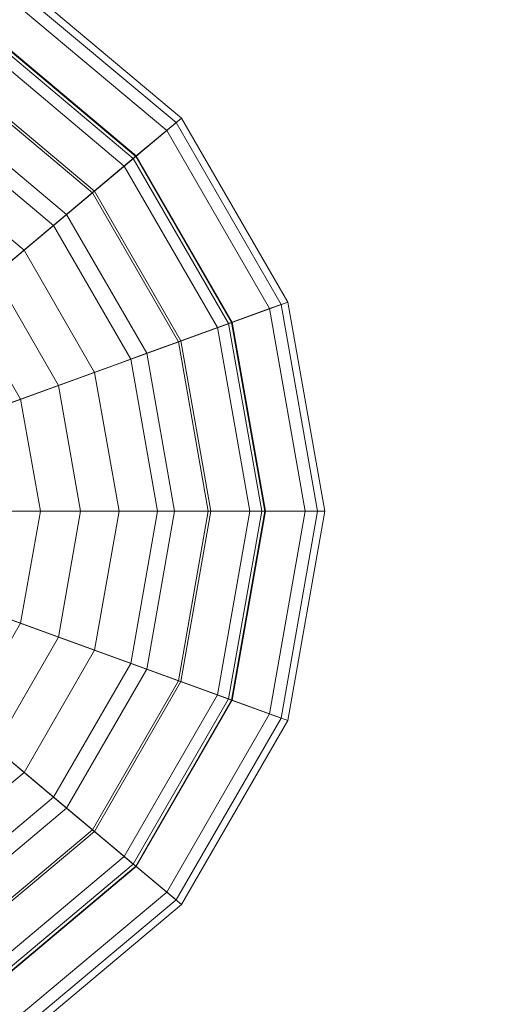
# Model space of a CAD drawing. Units: inches. Extents: x 375 to 1122, y 27 to 1069.
# Tile 142 of 155: x 733.741 to 734.829, y 898.026 to 900.205. Entities that reach past the tile are written whole.
import ezdxf

# ---------------------------------------------------------------- set-up
doc = ezdxf.new("R2010")
doc.units = ezdxf.units.IN
doc.layers.add('A-ANNO-DIMS', color=2, linetype='Continuous', lineweight=18)
doc.layers.add('Furniture', color=30, linetype='Continuous', lineweight=18)
doc.styles.get("Standard").update_dxf_attribs({"font": 'arial.ttf'})
doc.dimstyles.new('ISO-25', dxfattribs={"dimtxt": 12, "dimasz": 2.5, "dimexe": 1.5, "dimexo": 1.5, "dimtad": 1, "dimdec": 1, "dimlunit": 3, "dimtxsty": 'Standard', "dimblk": 'ARCHTICK', "dimcen": 2.5, "dimadec": 0, "dimazin": 0, "dimtfac": 1, "dimtdec": 1, "dimtmove": 0, "dimatfit": 3, "dimfxl": 1.5, "dimfxlon": 1, "dimarcsym": 0})

# ---------------------------------------------------------------- blocks, each defined once
blk = doc.blocks.new('A$C403C54AD')
for points in [[(0.980157, 1.23678, -0.04658), (0.980157, 1.202917, -0.043501), (0.980157, 1.202917, -0.043501), (0.968576, 1.234737, -0.04658)], [(0.980157, 1.233514, -0.043349), (0.980157, 1.23678, -0.04658), (0.968576, 1.234737, -0.04658), (0.969693, 1.231669, -0.043349)], [(0.991739, 1.234737, -0.04658), (0.980157, 1.202917, -0.043501), (0.980157, 1.202917, -0.043501), (0.980157, 1.23678, -0.04658)], [(0.990622, 1.231669, -0.043349), (0.991739, 1.234737, -0.04658), (0.980157, 1.23678, -0.04658), (0.980157, 1.233514, -0.043349)], [(0.980157, 1.233473, 0.116404), (0.980157, 1.236381, 0.10318), (0.968712, 1.234363, 0.10318), (0.969706, 1.231631, 0.116404)], [(0.980157, 1.236381, 0.10318), (0.980157, 1.235706, 0.074938), (0.968943, 1.233728, 0.074938), (0.968712, 1.234363, 0.10318)], [(0.990608, 1.231631, 0.116404), (0.991602, 1.234363, 0.10318), (0.980157, 1.236381, 0.10318), (0.980157, 1.233473, 0.116404)], [(0.991602, 1.234363, 0.10318), (0.991372, 1.233728, 0.074938), (0.980157, 1.235706, 0.074938), (0.980157, 1.236381, 0.10318)], [(0.980157, 1.235706, 0.074938), (0.980157, 1.230341, 0.056929), (0.970778, 1.228687, 0.056929), (0.968943, 1.233728, 0.074938)], [(0.991372, 1.233728, 0.074938), (0.989537, 1.228687, 0.056929), (0.980157, 1.230341, 0.056929), (0.980157, 1.235706, 0.074938)], [(0.968576, 1.234737, -0.04658), (0.980157, 1.202917, -0.043501), (0.980157, 1.202917, -0.043501), (0.958391, 1.228857, -0.04658)], [(0.969693, 1.231669, -0.043349), (0.968576, 1.234737, -0.04658), (0.958391, 1.228857, -0.04658), (0.96049, 1.226356, -0.043349)], [(1.001923, 1.228857, -0.04658), (0.980157, 1.202917, -0.043501), (0.980157, 1.202917, -0.043501), (0.991739, 1.234737, -0.04658)], [(0.999824, 1.226356, -0.043349), (1.001923, 1.228857, -0.04658), (0.991739, 1.234737, -0.04658), (0.990622, 1.231669, -0.043349)], [(0.969706, 1.231631, 0.116404), (0.968712, 1.234363, 0.10318), (0.958647, 1.228552, 0.10318), (0.960516, 1.226325, 0.116404)], [(0.968712, 1.234363, 0.10318), (0.968943, 1.233728, 0.074938), (0.959081, 1.228035, 0.074938), (0.958647, 1.228552, 0.10318)], [(0.999798, 1.226325, 0.116404), (1.001667, 1.228552, 0.10318), (0.991602, 1.234363, 0.10318), (0.990608, 1.231631, 0.116404)], [(1.001667, 1.228552, 0.10318), (1.001233, 1.228035, 0.074938), (0.991372, 1.233728, 0.074938), (0.991602, 1.234363, 0.10318)], [(0.968943, 1.233728, 0.074938), (0.970778, 1.228687, 0.056929), (0.96253, 1.223925, 0.056929), (0.959081, 1.228035, 0.074938)], [(0.980157, 1.217132, -0.040074), (0.980157, 1.233514, -0.043349), (0.969693, 1.231669, -0.043349), (0.975296, 1.216274, -0.040074)], [(0.980157, 1.228477, 0.12581), (0.980157, 1.233473, 0.116404), (0.969706, 1.231631, 0.116404), (0.971415, 1.226936, 0.12581)], [(0.980157, 1.233296, 0.102963), (0.980157, 1.230487, 0.115599), (0.970728, 1.228824, 0.115599), (0.969767, 1.231464, 0.102963)], [(0.980157, 1.232638, 0.075423), (0.980157, 1.233296, 0.102963), (0.969767, 1.231464, 0.102963), (0.969992, 1.230846, 0.075423)], [(0.985019, 1.216274, -0.040074), (0.990622, 1.231669, -0.043349), (0.980157, 1.233514, -0.043349), (0.980157, 1.217132, -0.040074)], [(0.988899, 1.226936, 0.12581), (0.990608, 1.231631, 0.116404), (0.980157, 1.233473, 0.116404), (0.980157, 1.228477, 0.12581)], [(0.990547, 1.231464, 0.102963), (0.989586, 1.228824, 0.115599), (0.980157, 1.230487, 0.115599), (0.980157, 1.233296, 0.102963)], [(0.990322, 1.230846, 0.075423), (0.990547, 1.231464, 0.102963), (0.980157, 1.233296, 0.102963), (0.980157, 1.232638, 0.075423)], [(1.001233, 1.228035, 0.074938), (0.997785, 1.223925, 0.056929), (0.989537, 1.228687, 0.056929), (0.991372, 1.233728, 0.074938)], [(0.980157, 1.227531, 0.058276), (0.980157, 1.232638, 0.075423), (0.969992, 1.230846, 0.075423), (0.971739, 1.226046, 0.058276)], [(0.988575, 1.226046, 0.058276), (0.990322, 1.230846, 0.075423), (0.980157, 1.232638, 0.075423), (0.980157, 1.227531, 0.058276)], [(0.975296, 1.216274, -0.040074), (0.969693, 1.231669, -0.043349), (0.96049, 1.226356, -0.043349), (0.971021, 1.213806, -0.040074)], [(0.989294, 1.213806, -0.040074), (0.999824, 1.226356, -0.043349), (0.990622, 1.231669, -0.043349), (0.985019, 1.216274, -0.040074)], [(0.971415, 1.226936, 0.12581), (0.969706, 1.231631, 0.116404), (0.960516, 1.226325, 0.116404), (0.963728, 1.222497, 0.12581)], [(0.969767, 1.231464, 0.102963), (0.970728, 1.228824, 0.115599), (0.962436, 1.224037, 0.115599), (0.96063, 1.226189, 0.102963)], [(0.969992, 1.230846, 0.075423), (0.969767, 1.231464, 0.102963), (0.96063, 1.226189, 0.102963), (0.961053, 1.225685, 0.075423)], [(0.996587, 1.222497, 0.12581), (0.999798, 1.226325, 0.116404), (0.990608, 1.231631, 0.116404), (0.988899, 1.226936, 0.12581)], [(0.999684, 1.226189, 0.102963), (0.997878, 1.224037, 0.115599), (0.989586, 1.228824, 0.115599), (0.990547, 1.231464, 0.102963)], [(0.999261, 1.225685, 0.075423), (0.999684, 1.226189, 0.102963), (0.990547, 1.231464, 0.102963), (0.990322, 1.230846, 0.075423)], [(0.971739, 1.226046, 0.058276), (0.969992, 1.230846, 0.075423), (0.961053, 1.225685, 0.075423), (0.964336, 1.221772, 0.058276)], [(0.995978, 1.221772, 0.058276), (0.999261, 1.225685, 0.075423), (0.990322, 1.230846, 0.075423), (0.988575, 1.226046, 0.058276)], [(0.980157, 1.230487, 0.115599), (0.980157, 1.225399, 0.12581), (0.972468, 1.224043, 0.12581), (0.970728, 1.228824, 0.115599)], [(0.980157, 1.230341, 0.056929), (0.980157, 1.223275, 0.046697), (0.973195, 1.222047, 0.046697), (0.970778, 1.228687, 0.056929)], [(0.989586, 1.228824, 0.115599), (0.987846, 1.224043, 0.12581), (0.980157, 1.225399, 0.12581), (0.980157, 1.230487, 0.115599)], [(0.989537, 1.228687, 0.056929), (0.98712, 1.222047, 0.046697), (0.980157, 1.223275, 0.046697), (0.980157, 1.230341, 0.056929)], [(0.958391, 1.228857, -0.04658), (0.980157, 1.202917, -0.043501), (0.980157, 1.202917, -0.043501), (0.950832, 1.219849, -0.04658)], [(0.96049, 1.226356, -0.043349), (0.958391, 1.228857, -0.04658), (0.950832, 1.219849, -0.04658), (0.95366, 1.218216, -0.043349)], [(0.960516, 1.226325, 0.116404), (0.958647, 1.228552, 0.10318), (0.951177, 1.219649, 0.10318), (0.953695, 1.218195, 0.116404)], [(0.958647, 1.228552, 0.10318), (0.959081, 1.228035, 0.074938), (0.951762, 1.219312, 0.074938), (0.951177, 1.219649, 0.10318)], [(0.970728, 1.228824, 0.115599), (0.972468, 1.224043, 0.12581), (0.965707, 1.220139, 0.12581), (0.962436, 1.224037, 0.115599)], [(0.970778, 1.228687, 0.056929), (0.973195, 1.222047, 0.046697), (0.967072, 1.218512, 0.046697), (0.96253, 1.223925, 0.056929)], [(0.980157, 1.225399, 0.12581), (0.980157, 1.228477, 0.12581), (0.971415, 1.226936, 0.12581), (0.972468, 1.224043, 0.12581)], [(1.009483, 1.219849, -0.04658), (0.980157, 1.202917, -0.043501), (0.980157, 1.202917, -0.043501), (1.001923, 1.228857, -0.04658)], [(0.987846, 1.224043, 0.12581), (0.988899, 1.226936, 0.12581), (0.980157, 1.228477, 0.12581), (0.980157, 1.225399, 0.12581)], [(0.997785, 1.223925, 0.056929), (0.993243, 1.218512, 0.046697), (0.98712, 1.222047, 0.046697), (0.989537, 1.228687, 0.056929)], [(0.997878, 1.224037, 0.115599), (0.994608, 1.220139, 0.12581), (0.987846, 1.224043, 0.12581), (0.989586, 1.228824, 0.115599)], [(1.00662, 1.218195, 0.116404), (1.009137, 1.219649, 0.10318), (1.001667, 1.228552, 0.10318), (0.999798, 1.226325, 0.116404)], [(1.006655, 1.218216, -0.043349), (1.009483, 1.219849, -0.04658), (1.001923, 1.228857, -0.04658), (0.999824, 1.226356, -0.043349)], [(1.009137, 1.219649, 0.10318), (1.008553, 1.219312, 0.074938), (1.001233, 1.228035, 0.074938), (1.001667, 1.228552, 0.10318)], [(0.959081, 1.228035, 0.074938), (0.96253, 1.223925, 0.056929), (0.956408, 1.216629, 0.056929), (0.951762, 1.219312, 0.074938)], [(1.008553, 1.219312, 0.074938), (1.003907, 1.216629, 0.056929), (0.997785, 1.223925, 0.056929), (1.001233, 1.228035, 0.074938)], [(0.980157, 1.221045, 0.048884), (0.980157, 1.227531, 0.058276), (0.971739, 1.226046, 0.058276), (0.973957, 1.219951, 0.048884)], [(0.986357, 1.219951, 0.048884), (0.988575, 1.226046, 0.058276), (0.980157, 1.227531, 0.058276), (0.980157, 1.221045, 0.048884)], [(0.972468, 1.224043, 0.12581), (0.971415, 1.226936, 0.12581), (0.963728, 1.222497, 0.12581), (0.965707, 1.220139, 0.12581)], [(0.994608, 1.220139, 0.12581), (0.996587, 1.222497, 0.12581), (0.988899, 1.226936, 0.12581), (0.987846, 1.224043, 0.12581)], [(0.971021, 1.213806, -0.040074), (0.96049, 1.226356, -0.043349), (0.95366, 1.218216, -0.043349), (0.967847, 1.210025, -0.040074)], [(0.963728, 1.222497, 0.12581), (0.960516, 1.226325, 0.116404), (0.953695, 1.218195, 0.116404), (0.958022, 1.215697, 0.12581)], [(0.992467, 1.210025, -0.040074), (1.006655, 1.218216, -0.043349), (0.999824, 1.226356, -0.043349), (0.989294, 1.213806, -0.040074)], [(1.002293, 1.215697, 0.12581), (1.00662, 1.218195, 0.116404), (0.999798, 1.226325, 0.116404), (0.996587, 1.222497, 0.12581)], [(0.96063, 1.226189, 0.102963), (0.962436, 1.224037, 0.115599), (0.956282, 1.216702, 0.115599), (0.953848, 1.218107, 0.102963)], [(0.961053, 1.225685, 0.075423), (0.96063, 1.226189, 0.102963), (0.953848, 1.218107, 0.102963), (0.954418, 1.217778, 0.075423)], [(0.964336, 1.221772, 0.058276), (0.961053, 1.225685, 0.075423), (0.954418, 1.217778, 0.075423), (0.958842, 1.215224, 0.058276)], [(0.973957, 1.219951, 0.048884), (0.971739, 1.226046, 0.058276), (0.964336, 1.221772, 0.058276), (0.968505, 1.216804, 0.048884)], [(0.991809, 1.216804, 0.048884), (0.995978, 1.221772, 0.058276), (0.988575, 1.226046, 0.058276), (0.986357, 1.219951, 0.048884)], [(1.001473, 1.215224, 0.058276), (1.005896, 1.217778, 0.075423), (0.999261, 1.225685, 0.075423), (0.995978, 1.221772, 0.058276)], [(1.006466, 1.218107, 0.102963), (1.004033, 1.216702, 0.115599), (0.997878, 1.224037, 0.115599), (0.999684, 1.226189, 0.102963)], [(1.005896, 1.217778, 0.075423), (1.006466, 1.218107, 0.102963), (0.999684, 1.226189, 0.102963), (0.999261, 1.225685, 0.075423)], [(0.962436, 1.224037, 0.115599), (0.965707, 1.220139, 0.12581), (0.960688, 1.214158, 0.12581), (0.956282, 1.216702, 0.115599)], [(1.004033, 1.216702, 0.115599), (0.999627, 1.214158, 0.12581), (0.994608, 1.220139, 0.12581), (0.997878, 1.224037, 0.115599)], [(0.96253, 1.223925, 0.056929), (0.967072, 1.218512, 0.046697), (0.962527, 1.213096, 0.046697), (0.956408, 1.216629, 0.056929)], [(1.003907, 1.216629, 0.056929), (0.997787, 1.213096, 0.046697), (0.993243, 1.218512, 0.046697), (0.997785, 1.223925, 0.056929)], [(0.980157, 1.223275, 0.046697), (0.980157, 1.213036, 0.03933), (0.976696, 1.212426, 0.03933), (0.973195, 1.222047, 0.046697)], [(0.98712, 1.222047, 0.046697), (0.983618, 1.212426, 0.03933), (0.980157, 1.213036, 0.03933), (0.980157, 1.223275, 0.046697)], [(0.965707, 1.220139, 0.12581), (0.963728, 1.222497, 0.12581), (0.958022, 1.215697, 0.12581), (0.960688, 1.214158, 0.12581)], [(0.999627, 1.214158, 0.12581), (1.002293, 1.215697, 0.12581), (0.996587, 1.222497, 0.12581), (0.994608, 1.220139, 0.12581)], [(0.973195, 1.222047, 0.046697), (0.976696, 1.212426, 0.03933), (0.973653, 1.210669, 0.03933), (0.967072, 1.218512, 0.046697)], [(0.993243, 1.218512, 0.046697), (0.986661, 1.210669, 0.03933), (0.983618, 1.212426, 0.03933), (0.98712, 1.222047, 0.046697)], [(0.968505, 1.216804, 0.048884), (0.964336, 1.221772, 0.058276), (0.958842, 1.215224, 0.058276), (0.964459, 1.211981, 0.048884)], [(0.995856, 1.211981, 0.048884), (1.001473, 1.215224, 0.058276), (0.995978, 1.221772, 0.058276), (0.991809, 1.216804, 0.048884)], [(0.980157, 1.211822, 0.042248), (0.980157, 1.221045, 0.048884), (0.973957, 1.219951, 0.048884), (0.977112, 1.211285, 0.042248)], [(0.983203, 1.211285, 0.042248), (0.986357, 1.219951, 0.048884), (0.980157, 1.221045, 0.048884), (0.980157, 1.211822, 0.042248)], [(0.977112, 1.211285, 0.042248), (0.973957, 1.219951, 0.048884), (0.968505, 1.216804, 0.048884), (0.974434, 1.209738, 0.042248)], [(0.985881, 1.209738, 0.042248), (0.991809, 1.216804, 0.048884), (0.986357, 1.219951, 0.048884), (0.983203, 1.211285, 0.042248)]]:
    blk.add_3dface(points)
blk = doc.blocks.new('_ArchTick')
at = {"color": 0, "linetype": 'ByBlock', "const_width": 0.15}
blk.add_lwpolyline([(-0.5, -0.5), (0.5, 0.5)], dxfattribs=at)
blk = doc.blocks.new('*D73')
at = {"layer": 'A-ANNO-DIMS', "color": 0, "lineweight": -2, "transparency": 16777216}
for p, q in [((686.7573, 932.4277), (686.7573, 929.4277)), ((770.7573, 932.4277), (770.7573, 929.4277)), ((686.7573, 930.9277), (770.7573, 930.9277)), ((770.7573, 930.9277), (987.6096, 930.9277))]:
    blk.add_line(p, q, dxfattribs=at)
at = {"layer": 'Defpoints', "color": 0, "transparency": 16777216}
for p in [(686.7573, 943.5277), (770.7573, 943.5277), (770.7573, 930.9277)]:
    blk.add_point(p, dxfattribs=at)
at = {"layer": 'A-ANNO-DIMS', "color": 0, "lineweight": -2, "transparency": 16777216, "xscale": 2.5, "yscale": 2.5, "zscale": 2.5, "rotation": 180}
blk.add_blockref('_ArchTick', (686.7573, 930.9277), dxfattribs=at)
at = {"layer": 'A-ANNO-DIMS', "color": 0, "lineweight": -2, "transparency": 16777216, "xscale": 2.5, "yscale": 2.5, "zscale": 2.5}
blk.add_blockref('_ArchTick', (770.7573, 930.9277), dxfattribs=at)
at = {"layer": 'A-ANNO-DIMS', "color": 0, "transparency": 16777216, "insert": (880.4335, 937.7573), "char_height": 12, "attachment_point": 5}
blk.add_mtext('2-PANEL SLIDER 7\'-0" TYP.', dxfattribs=at)
blk = doc.blocks.new('*D88')
at = {"layer": 'A-ANNO-DIMS', "color": 0, "lineweight": -2, "transparency": 16777216}
for p, q in [((731.0073, 1052.5277), (731.0073, 1055.5277)), ((854.0073, 1052.5277), (854.0073, 1055.5277)), ((731.0073, 1054.0277), (854.0073, 1054.0277))]:
    blk.add_line(p, q, dxfattribs=at)
at = {"layer": 'Defpoints', "color": 0, "transparency": 16777216}
for p in [(854.0073, 1054.0277), (731.0073, 502.5277), (854.0073, 502.5277)]:
    blk.add_point(p, dxfattribs=at)
at = {"layer": 'A-ANNO-DIMS', "color": 0, "lineweight": -2, "transparency": 16777216, "xscale": 2.5, "yscale": 2.5, "zscale": 2.5, "rotation": 180}
blk.add_blockref('_ArchTick', (731.0073, 1054.0277), dxfattribs=at)
at = {"layer": 'A-ANNO-DIMS', "color": 0, "lineweight": -2, "transparency": 16777216, "xscale": 2.5, "yscale": 2.5, "zscale": 2.5}
blk.add_blockref('_ArchTick', (854.0073, 1054.0277), dxfattribs=at)
at = {"layer": 'A-ANNO-DIMS', "color": 0, "transparency": 16777216, "insert": (792.5073, 1060.7837), "char_height": 12, "attachment_point": 5}
blk.add_mtext('10\'-3"', dxfattribs=at)
blk = doc.blocks.new('*D91')
at = {"layer": 'A-ANNO-DIMS', "color": 0, "lineweight": -2, "transparency": 16777216}
for p, q in [((728.0073, 1052.5277), (728.0073, 1055.5277)), ((788.0073, 1052.5277), (788.0073, 1055.5277)), ((728.0073, 1054.0277), (788.0073, 1054.0277))]:
    blk.add_line(p, q, dxfattribs=at)
at = {"layer": 'Defpoints', "color": 0, "transparency": 16777216}
for p in [(788.0073, 1054.0277), (728.0073, 774.0277), (788.0073, 774.0277)]:
    blk.add_point(p, dxfattribs=at)
at = {"layer": 'A-ANNO-DIMS', "color": 0, "lineweight": -2, "transparency": 16777216, "xscale": 2.5, "yscale": 2.5, "zscale": 2.5, "rotation": 180}
blk.add_blockref('_ArchTick', (728.0073, 1054.0277), dxfattribs=at)
at = {"layer": 'A-ANNO-DIMS', "color": 0, "lineweight": -2, "transparency": 16777216, "xscale": 2.5, "yscale": 2.5, "zscale": 2.5}
blk.add_blockref('_ArchTick', (788.0073, 1054.0277), dxfattribs=at)
at = {"layer": 'A-ANNO-DIMS', "color": 0, "transparency": 16777216, "insert": (758.0073, 1060.7796), "char_height": 12, "attachment_point": 5}
blk.add_mtext('5\'-0"', dxfattribs=at)

msp = doc.modelspace()

# ---------------------------------------------------------------- block references
at = {"layer": 'Furniture', "xscale": 39.9918517141215, "yscale": 39.9918517141215, "zscale": 39.9918517141215, "rotation": 270}
msp.add_blockref('A$C403C54AD', (684.9549, 938.3156, 0.024), dxfattribs=at)

# ---------------------------------------------------------------- dimensions: what is measured, and where the dimension line sits
at = {"layer": 'A-ANNO-DIMS'}
for base, p1, p2, picture, middle in [((788.0073, 1054.0277), (728.0073, 774.0277), (788.0073, 774.0277), '*D91', (758.0073, 1060.7796)), ((854.0073, 1054.0277), (731.0073, 502.5277), (854.0073, 502.5277), '*D88', (792.5073, 1060.7837))]:
    dim = msp.add_linear_dim(base=base, p1=p1, p2=p2, dimstyle='ISO-25', override={"dimdec": 1, "dimlfac": 1, "dimrnd": 0, "dimzin": 1, "dimdsep": 46, "dimlunit": 4, "dimfrac": 2}, dxfattribs=at)
    dim.commit()
    dim.dimension.update_dxf_attribs({"geometry": picture, "text_midpoint": middle})
dim = msp.add_linear_dim(base=(770.7573, 930.9277), p1=(686.7573, 943.5277), p2=(770.7573, 943.5277), text='2-PANEL SLIDER <> TYP.', dimstyle='ISO-25', override={"dimdec": 1, "dimlfac": 1, "dimrnd": 0, "dimzin": 1, "dimdsep": 46, "dimlunit": 4, "dimfrac": 2}, dxfattribs=at)
dim.commit()
dim.dimension.update_dxf_attribs({"geometry": '*D73', "text_midpoint": (880.4335, 937.7573)})

doc.saveas('drawing.dxf')
